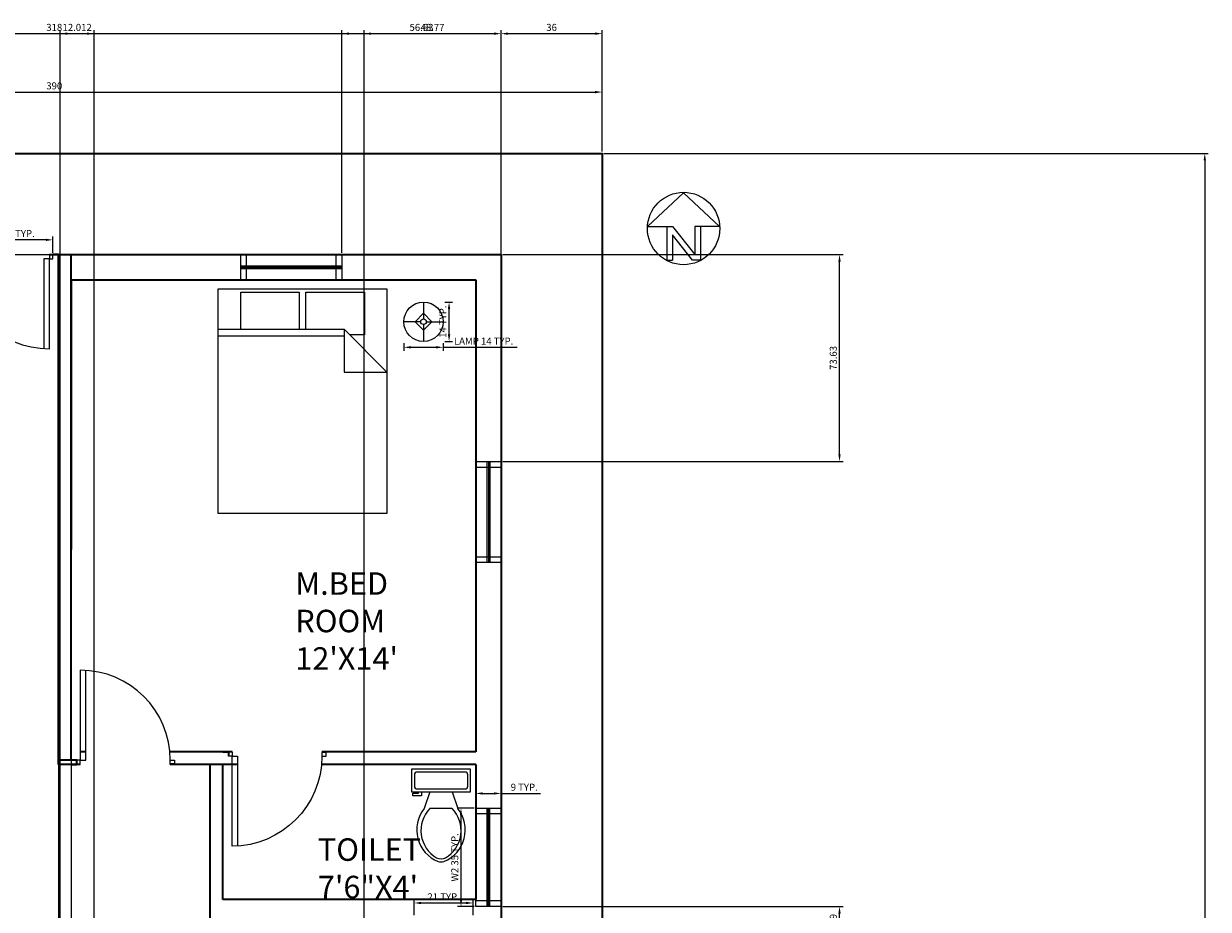
# Model space of a CAD drawing. Units: inches. Extents: x 204 to 942, y 1794 to 2670.
# Tile 6 of 6: x 521 to 942, y 2355 to 2670. Entities that reach past the tile are written whole.
import ezdxf

# ---------------------------------------------------------------- set-up
doc = ezdxf.new("R2010")
doc.units = ezdxf.units.IN
for name, color, linetype, lineweight in [('A-ANNO-DIMS', 2, 'Continuous', 18), ('A-ANNO-SYMB', 7, 'Continuous', 25), ('A-AREA-IDEN', 7, 'Continuous', 18), ('A-DOOR', 3, 'Continuous', 18), ('A-FLOR-FIXT', 9, 'Continuous', 18), ('A-FLOR-OTLN', 7, 'Continuous', 25), ('A-FURN', 8, 'Continuous', 18), ('A-GLAZ', 4, 'Continuous', 18), ('A-WALL', 7, 'Continuous', 35), ('C-PROP', 7, 'Continuous', 35)]:
    doc.layers.add(name, color=color, linetype=linetype, lineweight=lineweight)
doc.styles.get("Standard").update_dxf_attribs({"font": 'arial.ttf'})
doc.dimstyles.new('ISO-25', dxfattribs={"dimtxt": 2.5, "dimasz": 2.5, "dimexe": 1.25, "dimexo": 0.625, "dimtad": 1, "dimtxsty": 'Standard', "dimcen": 2.5, "dimadec": 0, "dimazin": 0, "dimtfac": 1, "dimtmove": 0, "dimatfit": 3, "dimfxl": 1, "dimarcsym": 0})

# ---------------------------------------------------------------- blocks, each defined once
blk = doc.blocks.new('Bed - Queen')
for p, q in [((0, -80.00003), (0, 0)), ((0, 0), (59.99999, 0)), ((59.99999, 0), (59.99999, -80.00003)), ((7.99999, -1.2), (28.79998, -1.2)), ((7.99999, -14.4), (7.99999, -1.2)), ((28.79998, -1.2), (28.79998, -14.4)), ((31.19999, -1.2), (51.99999, -1.2)), ((31.19999, -14.4), (31.19999, -1.2)), ((51.99999, -1.2), (51.99999, -16.4)), ((0, -14.4), (44.8, -14.4)), ((44.8, -16.8), (0, -16.8)), ((59.99999, -29.6), (44.8, -14.4)), ((44.8, -14.4), (44.8, -29.6)), ((51.99999, -16.4), (46.79936, -16.4)), ((44.8, -29.6), (59.99999, -29.6)), ((59.99999, -80.00003), (0, -80.00003))]:
    blk.add_line(p, q)
blk = doc.blocks.new('Lamp - Table')
for p, q in [((0, 7), (0, 1)), ((-1, 0), (-7, 0)), ((0, 3), (-3, 0)), ((-3, 0), (0, -3)), ((3, 0), (0, 3)), ((0, -3), (3, 0)), ((1, 0), (7, 0)), ((0, -1), (0, -7))]:
    blk.add_line(p, q)
for radius in [7, 1]:
    blk.add_circle((0, 0), radius)
blk = doc.blocks.new('Toilet - top')
for p, q in [((9.5, -6), (9.5, -2)), ((-8, -8.5), (-8, -8)), ((-7, -8), (-7, -9.5)), ((-4, -8), (-6, -14)), ((4, -8), (6, -14)), ((-10, -8.5), (-8, -8.5)), ((-10, -9.5), (-10, -8.5)), ((-7, -9.5), (-10, -9.5)), ((4, -14), (-4, -14))]:
    blk.add_line(p, q)
blk.add_lwpolyline([(10.5, -8), (10.5, 0), (-10.5, 0), (-10.5, -8)], close=True)
for points in [[(-9.5, -2), (-9.5, -6)], [(8.5, -1), (-8.5, -1)], [(-8.5, -7), (8.5, -7)]]:
    blk.add_lwpolyline(points)
for centre, radius, start, end in [((-8.62, -1.88), 0.884, 81.8699, 188.1301), ((8.62, -1.88), 0.884, 351.8699, 98.1301), ((-8.62, -6.12), 0.884, 171.8699, 278.1301), ((8.62, -6.12), 0.884, 261.8699, 8.1301), ((3.52, -21.58), 12.17, 141.4691, 247.9714), ((4.2, -21.82), 11.33, 136.3677, 238.9468), ((-3.52, -21.58), 12.17, 292.0284, 38.5307), ((-4.2, -21.82), 11.33, 301.053, 43.6321), ((0, -27.88), 4, 245.7318, 294.2682), ((0, -29), 4, 254.8605, 285.1395)]:
    blk.add_arc(centre, radius, start, end)
blk = doc.blocks.new('North Arrow')
for p, q in [((0, 0), (-12.86, -11.999)), ((0, 0), (12.782, -11.999)), ((-12.86, -11.999), (-6, -11.999)), ((-6, -11.999), (-6, -23.999)), ((-6, -11.999), (-4, -11.999)), ((-4, -11.999), (4, -21.999)), ((4, -11.999), (4, -21.999)), ((6, -11.999), (4, -11.999)), ((12.782, -11.999), (6, -11.999)), ((6, -11.999), (6, -23.999)), ((3.195, -23.996), (-4, -15.002)), ((-4, -15.002), (-4, -23.999)), ((-6, -23.999), (-4, -23.999)), ((6, -23.999), (3.195, -23.999))]:
    blk.add_line(p, q)
blk.add_circle((-0.013, -12.745), 12.885)
blk = doc.blocks.new('*D10')
at = {"layer": 'A-ANNO-DIMS', "color": 0, "lineweight": -2, "transparency": 16777216}
for p, q in [((336.74, 2624.88), (336.74, 2647.31)), ((339.24, 2646.06), (724.24, 2646.06)), ((726.74, 2624.88), (726.74, 2647.31))]:
    blk.add_line(p, q, dxfattribs=at)
at = {"layer": 'A-ANNO-DIMS', "color": 0, "transparency": 16777216}
for points in [[(339.24, 2646.47), (339.24, 2645.64), (336.74, 2646.06)], [(724.24, 2646.47), (724.24, 2645.64), (726.74, 2646.06)]]:
    blk.add_solid(points, dxfattribs=at)
at = {"layer": 'Defpoints', "color": 0, "transparency": 16777216}
for p in [(726.74, 2646.06), (336.74, 2624.26), (726.74, 2624.26)]:
    blk.add_point(p, dxfattribs=at)
at = {"layer": 'A-ANNO-DIMS', "color": 0, "transparency": 16777216, "insert": (531.74, 2647.96), "char_height": 2.5, "attachment_point": 5}
blk.add_mtext('390', dxfattribs=at)
blk = doc.blocks.new('*D12')
at = {"layer": 'A-ANNO-DIMS', "color": 0, "lineweight": -2, "transparency": 16777216}
for p, q in [((727.37, 2624.26), (942.46, 2624.26)), ((941.21, 2621.76), (941.21, 1840.76)), ((727.37, 1838.26), (942.46, 1838.26))]:
    blk.add_line(p, q, dxfattribs=at)
at = {"layer": 'A-ANNO-DIMS', "color": 0, "transparency": 16777216}
for points in [[(940.79, 2621.76), (941.63, 2621.76), (941.21, 2624.26)], [(940.79, 1840.76), (941.63, 1840.76), (941.21, 1838.26)]]:
    blk.add_solid(points, dxfattribs=at)
at = {"layer": 'Defpoints', "color": 0, "transparency": 16777216}
for p in [(726.74, 2624.26), (726.74, 1838.26), (941.21, 1838.26)]:
    blk.add_point(p, dxfattribs=at)
at = {"layer": 'A-ANNO-DIMS', "color": 0, "transparency": 16777216, "insert": (939.31, 2231.26), "char_height": 2.5, "attachment_point": 5, "rotation": 90}
blk.add_mtext('786', dxfattribs=at)
blk = doc.blocks.new('WIN-36IN')
for p, q in [((0, 9), (36, 9)), ((0, 0), (0, 9)), ((2, 0), (2, 9)), ((34, 0), (34, 9)), ((36, 9), (36, 0)), ((0, 5), (36, 5)), ((0, 4.5), (36, 4.5)), ((0, 4), (36, 4)), ((36, 0), (0, 0)), ((0, 0), (2, 0)), ((36, 0), (34, 0))]:
    blk.add_line(p, q)
blk = doc.blocks.new('WIN-35IN')
for p, q in [((0, 0), (0, 35)), ((0, 35), (9, 35)), ((4, 0), (4, 35)), ((4.5, 0), (4.5, 35)), ((5, 0), (5, 35)), ((9, 35), (9, 0)), ((9, 35), (9, 33)), ((9, 33), (0, 33)), ((9, 2), (0, 2)), ((9, 0), (0, 0)), ((9, 0), (9, 2))]:
    blk.add_line(p, q)
blk = doc.blocks.new('DOOR-SWING-32IN')
for p, q in [((3.26, 1.55), (3.26, 33.49)), ((1.26, 1.55), (3.26, 1.55))]:
    blk.add_line(p, q)
blk.add_lwpolyline([(1.26, 33.55), (1.26, 1.55), (3.26, 1.55)])
for points in [[(1.26, 1.55), (0, 1.55), (0, 0), (1.26, 0)], [(33.26, 1.55), (34.79, 1.55), (34.79, 0.26), (33.26, 0.26)]]:
    blk.add_lwpolyline(points, close=True)
blk.add_arc((1.26, 1.55), 32, 0, 90)
blk = doc.blocks.new('*D16')
at = {"layer": 'A-ANNO-DIMS', "color": 0, "lineweight": -2, "transparency": 16777216}
for p, q in [((496.46, 2588.88), (496.46, 2594.73)), ((528.74, 2593.48), (498.96, 2593.48)), ((531.24, 2588.88), (531.24, 2594.73))]:
    blk.add_line(p, q, dxfattribs=at)
at = {"layer": 'A-ANNO-DIMS', "color": 0, "transparency": 16777216}
for points in [[(498.96, 2593.89), (498.96, 2593.06), (496.46, 2593.48)], [(528.74, 2593.89), (528.74, 2593.06), (531.24, 2593.48)]]:
    blk.add_solid(points, dxfattribs=at)
at = {"layer": 'Defpoints', "color": 0, "transparency": 16777216}
for p in [(496.46, 2593.48), (496.46, 2588.26), (531.24, 2588.26)]:
    blk.add_point(p, dxfattribs=at)
at = {"layer": 'A-ANNO-DIMS', "color": 0, "transparency": 16777216, "insert": (513.85, 2595.4), "char_height": 2.5, "attachment_point": 5}
blk.add_mtext('DOOR 35 TYP.', dxfattribs=at)
blk = doc.blocks.new('*D20')
at = {"layer": 'A-ANNO-DIMS', "color": 0, "lineweight": -2, "transparency": 16777216}
for p, q in [((681.13, 2391.22), (675.26, 2391.22)), ((676.51, 2358.72), (676.51, 2388.72)), ((681.13, 2356.22), (675.26, 2356.22))]:
    blk.add_line(p, q, dxfattribs=at)
at = {"layer": 'A-ANNO-DIMS', "color": 0, "transparency": 16777216}
for points in [[(676.09, 2388.72), (676.92, 2388.72), (676.51, 2391.22)], [(676.09, 2358.72), (676.92, 2358.72), (676.51, 2356.22)]]:
    blk.add_solid(points, dxfattribs=at)
at = {"layer": 'Defpoints', "color": 0, "transparency": 16777216}
for p in [(676.51, 2391.22), (681.76, 2391.22), (681.76, 2356.22)]:
    blk.add_point(p, dxfattribs=at)
at = {"layer": 'A-ANNO-DIMS', "color": 0, "transparency": 16777216, "insert": (674.6, 2373.72), "char_height": 2.5, "attachment_point": 5, "rotation": 90}
blk.add_mtext('W2 35 TYP.', dxfattribs=at)
blk = doc.blocks.new('*D21')
at = {"layer": 'A-ANNO-DIMS', "color": 0, "lineweight": -2, "transparency": 16777216}
for p, q in [((681.76, 2391.85), (681.76, 2397.72)), ((684.26, 2396.47), (688.26, 2396.47)), ((690.76, 2391.85), (690.76, 2397.72)), ((690.76, 2396.47), (704.73, 2396.47))]:
    blk.add_line(p, q, dxfattribs=at)
at = {"layer": 'A-ANNO-DIMS', "color": 0, "transparency": 16777216}
for points in [[(684.26, 2396.89), (684.26, 2396.05), (681.76, 2396.47)], [(688.26, 2396.89), (688.26, 2396.05), (690.76, 2396.47)]]:
    blk.add_solid(points, dxfattribs=at)
at = {"layer": 'Defpoints', "color": 0, "transparency": 16777216}
for p in [(690.76, 2396.47), (681.76, 2391.22), (690.76, 2391.22)]:
    blk.add_point(p, dxfattribs=at)
at = {"layer": 'A-ANNO-DIMS', "color": 0, "transparency": 16777216, "insert": (698.99, 2398.37), "char_height": 2.5, "attachment_point": 5}
blk.add_mtext('9 TYP.', dxfattribs=at)
blk = doc.blocks.new('*D24')
at = {"layer": 'A-ANNO-DIMS', "color": 0, "lineweight": -2, "transparency": 16777216}
for p, q in [((656.15, 2556.71), (656.15, 2553.99)), ((658.65, 2555.24), (667.65, 2555.24)), ((670.15, 2556.71), (670.15, 2553.99)), ((670.15, 2555.24), (696.44, 2555.24))]:
    blk.add_line(p, q, dxfattribs=at)
at = {"layer": 'A-ANNO-DIMS', "color": 0, "transparency": 16777216}
for points in [[(658.65, 2555.65), (658.65, 2554.82), (656.15, 2555.24)], [(667.65, 2555.65), (667.65, 2554.82), (670.15, 2555.24)]]:
    blk.add_solid(points, dxfattribs=at)
at = {"layer": 'Defpoints', "color": 0, "transparency": 16777216}
for p in [(656.15, 2557.34), (670.15, 2557.34), (670.15, 2555.24)]:
    blk.add_point(p, dxfattribs=at)
at = {"layer": 'A-ANNO-DIMS', "color": 0, "transparency": 16777216, "insert": (684.54, 2557.12), "char_height": 2.5, "attachment_point": 5}
blk.add_mtext('LAMP 14 TYP.', dxfattribs=at)
blk = doc.blocks.new('*D25')
at = {"layer": 'A-ANNO-DIMS', "color": 0, "lineweight": -2, "transparency": 16777216}
for p, q in [((670.77, 2571.34), (673.5, 2571.34)), ((672.25, 2559.84), (672.25, 2568.84)), ((670.77, 2557.34), (673.5, 2557.34))]:
    blk.add_line(p, q, dxfattribs=at)
at = {"layer": 'A-ANNO-DIMS', "color": 0, "transparency": 16777216}
for points in [[(671.83, 2568.84), (672.67, 2568.84), (672.25, 2571.34)], [(671.83, 2559.84), (672.67, 2559.84), (672.25, 2557.34)]]:
    blk.add_solid(points, dxfattribs=at)
at = {"layer": 'Defpoints', "color": 0, "transparency": 16777216}
for p in [(670.15, 2571.34), (672.25, 2571.34), (670.15, 2557.34)]:
    blk.add_point(p, dxfattribs=at)
at = {"layer": 'A-ANNO-DIMS', "color": 0, "transparency": 16777216, "insert": (670.37, 2564.34), "char_height": 2.5, "attachment_point": 5, "rotation": 90}
blk.add_mtext('14 TYP.', dxfattribs=at)
blk = doc.blocks.new('*D27')
at = {"layer": 'A-ANNO-DIMS', "color": 0, "lineweight": -2, "transparency": 16777216}
for p, q in [((659.8, 2353.16), (659.8, 2358.74)), ((662.3, 2357.49), (678.3, 2357.49)), ((680.8, 2353.16), (680.8, 2358.74))]:
    blk.add_line(p, q, dxfattribs=at)
at = {"layer": 'A-ANNO-DIMS', "color": 0, "transparency": 16777216}
for points in [[(662.3, 2357.91), (662.3, 2357.07), (659.8, 2357.49)], [(678.3, 2357.91), (678.3, 2357.07), (680.8, 2357.49)]]:
    blk.add_solid(points, dxfattribs=at)
at = {"layer": 'Defpoints', "color": 0, "transparency": 16777216}
for p in [(680.8, 2357.49), (659.8, 2352.53), (680.8, 2352.53)]:
    blk.add_point(p, dxfattribs=at)
at = {"layer": 'A-ANNO-DIMS', "color": 0, "transparency": 16777216, "insert": (670.3, 2359.37), "char_height": 2.5, "attachment_point": 5}
blk.add_mtext('21 TYP.', dxfattribs=at)
blk = doc.blocks.new('*D38')
at = {"layer": 'A-ANNO-DIMS', "color": 0, "lineweight": -2, "transparency": 16777216}
for p, q in [((372.74, 2624.88), (372.74, 2668.11)), ((375.24, 2666.86), (688.24, 2666.86)), ((690.74, 2624.88), (690.74, 2668.11))]:
    blk.add_line(p, q, dxfattribs=at)
at = {"layer": 'A-ANNO-DIMS', "color": 0, "transparency": 16777216}
for points in [[(375.24, 2667.28), (375.24, 2666.44), (372.74, 2666.86)], [(688.24, 2667.28), (688.24, 2666.44), (690.74, 2666.86)]]:
    blk.add_solid(points, dxfattribs=at)
at = {"layer": 'Defpoints', "color": 0, "transparency": 16777216}
for p in [(690.74, 2666.86), (372.74, 2624.26), (690.74, 2624.26)]:
    blk.add_point(p, dxfattribs=at)
at = {"layer": 'A-ANNO-DIMS', "color": 0, "transparency": 16777216, "insert": (531.74, 2668.76), "char_height": 2.5, "attachment_point": 5}
blk.add_mtext('318', dxfattribs=at)
blk = doc.blocks.new('*D41')
at = {"layer": 'A-ANNO-DIMS', "color": 0, "lineweight": -2, "transparency": 16777216}
for p, q in [((690.74, 2588.88), (690.74, 2668.11)), ((693.24, 2666.86), (724.24, 2666.86)), ((726.74, 2624.88), (726.74, 2668.11))]:
    blk.add_line(p, q, dxfattribs=at)
at = {"layer": 'A-ANNO-DIMS', "color": 0, "transparency": 16777216}
for points in [[(693.24, 2667.28), (693.24, 2666.44), (690.74, 2666.86)], [(724.24, 2667.28), (724.24, 2666.44), (726.74, 2666.86)]]:
    blk.add_solid(points, dxfattribs=at)
at = {"layer": 'Defpoints', "color": 0, "transparency": 16777216}
for p in [(726.74, 2666.86), (726.74, 2624.26), (690.74, 2588.26)]:
    blk.add_point(p, dxfattribs=at)
at = {"layer": 'A-ANNO-DIMS', "color": 0, "transparency": 16777216, "insert": (708.74, 2668.76), "char_height": 2.5, "attachment_point": 5}
blk.add_mtext('36', dxfattribs=at)
blk = doc.blocks.new('*D47')
at = {"layer": 'A-ANNO-DIMS', "color": 0, "lineweight": -2, "transparency": 16777216}
for p, q in [((533.86, 2137.88), (533.86, 2668.11)), ((536.36, 2666.86), (543.38, 2666.86)), ((545.88, 2137.88), (545.88, 2668.11))]:
    blk.add_line(p, q, dxfattribs=at)
at = {"layer": 'A-ANNO-DIMS', "color": 0, "transparency": 16777216}
for points in [[(536.36, 2667.28), (536.36, 2666.44), (533.86, 2666.86)], [(543.38, 2667.28), (543.38, 2666.44), (545.88, 2666.86)]]:
    blk.add_solid(points, dxfattribs=at)
at = {"layer": 'Defpoints', "color": 0, "transparency": 16777216}
for p in [(545.88, 2666.86), (533.86, 2137.26), (545.88, 2137.26)]:
    blk.add_point(p, dxfattribs=at)
at = {"layer": 'A-ANNO-DIMS', "color": 0, "transparency": 16777216, "insert": (539.87, 2668.76), "char_height": 2.5, "attachment_point": 5}
blk.add_mtext('12.012', dxfattribs=at)
blk = doc.blocks.new('*D48')
at = {"layer": 'A-ANNO-DIMS', "color": 0, "lineweight": -2, "transparency": 16777216}
for p, q in [((641.98, 2014.8), (641.98, 2668.11)), ((644.48, 2666.86), (688.24, 2666.86)), ((690.74, 2014.8), (690.74, 2668.11))]:
    blk.add_line(p, q, dxfattribs=at)
at = {"layer": 'A-ANNO-DIMS', "color": 0, "transparency": 16777216}
for points in [[(644.48, 2667.28), (644.48, 2666.44), (641.98, 2666.86)], [(688.24, 2667.28), (688.24, 2666.44), (690.74, 2666.86)]]:
    blk.add_solid(points, dxfattribs=at)
at = {"layer": 'Defpoints', "color": 0, "transparency": 16777216}
for p in [(690.74, 2666.86), (641.98, 2014.18), (690.74, 2014.18)]:
    blk.add_point(p, dxfattribs=at)
at = {"layer": 'A-ANNO-DIMS', "color": 0, "transparency": 16777216, "insert": (666.36, 2668.76), "char_height": 2.5, "attachment_point": 5}
blk.add_mtext('48.77', dxfattribs=at)
blk = doc.blocks.new('*D50')
at = {"layer": 'A-ANNO-DIMS', "color": 0, "lineweight": -2, "transparency": 16777216}
for p, q in [((533.24, 2587.63), (533.24, 1794.41)), ((537.74, 2578.63), (537.74, 1794.41)), ((530.74, 1795.66), (528.24, 1795.66)), ((533.24, 1795.66), (537.74, 1795.66)), ((540.24, 1795.66), (548.67, 1795.66))]:
    blk.add_line(p, q, dxfattribs=at)
at = {"layer": 'A-ANNO-DIMS', "color": 0, "transparency": 16777216}
for points in [[(530.74, 1796.08), (530.74, 1795.24), (533.24, 1795.66)], [(540.24, 1796.08), (540.24, 1795.24), (537.74, 1795.66)]]:
    blk.add_solid(points, dxfattribs=at)
at = {"layer": 'Defpoints', "color": 0, "transparency": 16777216}
for p in [(533.24, 2588.26), (537.74, 2579.26), (537.74, 1795.66)]:
    blk.add_point(p, dxfattribs=at)
at = {"layer": 'A-ANNO-DIMS', "color": 0, "transparency": 16777216, "insert": (545.7, 1797.56), "char_height": 2.5, "attachment_point": 5}
blk.add_mtext('4.5', dxfattribs=at)
blk = doc.blocks.new('*D53')
at = {"layer": 'A-ANNO-DIMS', "color": 0, "lineweight": -2, "transparency": 16777216}
for p, q in [((634.11, 2588.9), (634.11, 2668.11)), ((636.61, 2666.86), (688.24, 2666.86)), ((690.74, 2588.88), (690.74, 2668.11))]:
    blk.add_line(p, q, dxfattribs=at)
at = {"layer": 'A-ANNO-DIMS', "color": 0, "transparency": 16777216}
for points in [[(636.61, 2667.28), (636.61, 2666.44), (634.11, 2666.86)], [(688.24, 2667.28), (688.24, 2666.44), (690.74, 2666.86)]]:
    blk.add_solid(points, dxfattribs=at)
at = {"layer": 'Defpoints', "color": 0, "transparency": 16777216}
for p in [(690.74, 2666.86), (634.11, 2588.28), (690.74, 2588.26)]:
    blk.add_point(p, dxfattribs=at)
at = {"layer": 'A-ANNO-DIMS', "color": 0, "transparency": 16777216, "insert": (662.43, 2668.76), "char_height": 2.5, "attachment_point": 5}
blk.add_mtext('56.63', dxfattribs=at)
blk = doc.blocks.new('*D59')
at = {"layer": 'A-ANNO-DIMS', "color": 0, "lineweight": -2, "transparency": 16777216}
for p, q in [((691.37, 2588.26), (812.46, 2588.26)), ((811.21, 2517.13), (811.21, 2585.76)), ((691.35, 2514.63), (812.46, 2514.63))]:
    blk.add_line(p, q, dxfattribs=at)
at = {"layer": 'A-ANNO-DIMS', "color": 0, "transparency": 16777216}
for points in [[(810.79, 2585.76), (811.62, 2585.76), (811.21, 2588.26)], [(810.79, 2517.13), (811.62, 2517.13), (811.21, 2514.63)]]:
    blk.add_solid(points, dxfattribs=at)
at = {"layer": 'Defpoints', "color": 0, "transparency": 16777216}
for p in [(690.74, 2588.26), (811.21, 2588.26), (690.72, 2514.63)]:
    blk.add_point(p, dxfattribs=at)
at = {"layer": 'A-ANNO-DIMS', "color": 0, "transparency": 16777216, "insert": (809.31, 2551.45), "char_height": 2.5, "attachment_point": 5, "rotation": 90}
blk.add_mtext('73.63', dxfattribs=at)
blk = doc.blocks.new('*D61')
at = {"layer": 'A-ANNO-DIMS', "color": 0, "lineweight": -2, "transparency": 16777216}
for p, q in [((691.38, 2356.22), (812.46, 2356.22)), ((811.21, 2344.93), (811.21, 2353.72)), ((691.38, 2342.43), (812.46, 2342.43))]:
    blk.add_line(p, q, dxfattribs=at)
at = {"layer": 'A-ANNO-DIMS', "color": 0, "transparency": 16777216}
for points in [[(810.79, 2353.72), (811.62, 2353.72), (811.21, 2356.22)], [(810.79, 2344.93), (811.62, 2344.93), (811.21, 2342.43)]]:
    blk.add_solid(points, dxfattribs=at)
at = {"layer": 'Defpoints', "color": 0, "transparency": 16777216}
for p in [(690.76, 2356.22), (811.21, 2356.22), (690.75, 2342.43)]:
    blk.add_point(p, dxfattribs=at)
at = {"layer": 'A-ANNO-DIMS', "color": 0, "transparency": 16777216, "insert": (809.31, 2349.33), "char_height": 2.5, "attachment_point": 5, "rotation": 90}
blk.add_mtext('13.79', dxfattribs=at)

msp = doc.modelspace()

# ---------------------------------------------------------------- linework, layer by layer
at = {"layer": 'A-FLOR-OTLN'}
msp.add_lwpolyline([(372.7443, 2588.2597), (690.7443, 2588.2597), (690.7443, 2138.2597), (372.7443, 2138.2597)], close=True, dxfattribs=at)
at = {"layer": 'A-WALL'}
for p, q in [((529.9822, 2588.2597), (537.7443, 2588.2597)), ((533.2443, 2588.2597), (531.2443, 2588.2597)), ((533.2443, 2588.2597), (690.7443, 2588.2597)), ((533.2443, 2579.2597), (533.2443, 2588.2597)), ((537.7443, 2579.2597), (537.7443, 2588.2597)), ((537.7443, 2588.2597), (539.7443, 2588.2597)), ((539.7443, 2588.2597), (548.9949, 2588.2597)), ((690.7443, 2588.2597), (690.7443, 2411.2597)), ((533.2443, 2579.2597), (533.2443, 2483.2597)), ((533.2443, 2411.2597), (533.2443, 2579.2597)), ((537.7443, 2579.2597), (537.7443, 2483.2597)), ((537.7443, 2579.2597), (681.7443, 2579.2597)), ((537.7443, 2411.2597), (537.7443, 2579.2597)), ((681.7443, 2579.2597), (681.7443, 2411.2597)), ((533.2443, 2406.7597), (533.2443, 2478.7597)), ((533.2443, 2406.7597), (533.2443, 2478.7597)), ((537.7443, 2408.3112), (537.7443, 2478.7597)), ((537.7443, 2408.3112), (537.7443, 2478.7597)), ((539.7443, 2408.3112), (533.2443, 2408.3112)), ((539.7443, 2406.7597), (539.7443, 2408.3112)), ((543.0064, 2411.2597), (541.0064, 2411.2597)), ((595.0064, 2411.2597), (572.8703, 2411.2597)), ((591.7443, 2411.2597), (593.7443, 2411.2597)), ((593.7443, 2411.2597), (593.7443, 2409.7082)), ((681.7443, 2411.2597), (626.9688, 2411.2597)), ((690.7443, 2411.2597), (690.7443, 2330.2597)), ((537.7443, 2406.7597), (533.2443, 2406.7597)), ((537.7443, 2406.7597), (539.7443, 2406.7597)), ((541.0064, 2406.7597), (537.7443, 2406.7597)), ((573.0064, 2407.0155), (573.0064, 2406.7597)), ((597.0064, 2406.7597), (573.0064, 2406.7597)), ((587.2443, 2358.7597), (587.2443, 2406.7597)), ((591.7443, 2358.7597), (591.7443, 2406.7597)), ((681.7443, 2406.7597), (626.8703, 2406.7597)), ((681.7443, 2406.7597), (681.7443, 2358.7597)), ((587.2443, 2341.4841), (587.2443, 2358.7597)), ((681.7443, 2358.7597), (591.7443, 2358.7597)), ((681.7443, 2358.7597), (591.7443, 2358.7597))]:
    msp.add_line(p, q, dxfattribs=at)
at = {"layer": 'C-PROP'}
for p, q in [((533.2443, 2624.2597), (690.7443, 2624.2597)), ((726.7443, 2588.2597), (726.7443, 2411.2597))]:
    msp.add_line(p, q, dxfattribs=at)
msp.add_lwpolyline([(336.7443, 2102.2597), (336.7443, 2624.2597), (726.7443, 2624.2597), (726.7443, 2102.2597)], dxfattribs=at)

# ---------------------------------------------------------------- block references
at = {"layer": 'A-ANNO-SYMB'}
msp.add_blockref('North Arrow', (755.7363, 2610.2578), dxfattribs=at)
at = {"layer": 'A-DOOR', "rotation": 180}
msp.add_blockref('DOOR-SWING-32IN', (531.2446, 2588.2593), dxfattribs=at)
at = {"layer": 'A-DOOR'}
msp.add_blockref('DOOR-SWING-32IN', (539.744, 2406.76), dxfattribs=at)
at = {"layer": 'A-DOOR', "extrusion": (0, 0, -1), "zscale": -1, "rotation": 180}
msp.add_blockref('DOOR-SWING-32IN', (-593.744, 2411.2593), dxfattribs=at)
at = {"layer": 'A-FLOR-FIXT'}
msp.add_blockref('Toilet - top', (669.3848, 2405.0832), dxfattribs=at)
at = {"layer": 'A-FURN'}
for name, p in [('Bed - Queen', (590.1138, 2576.0464)), ('Lamp - Table', (663.1483, 2564.3369))]:
    msp.add_blockref(name, p, dxfattribs=at)
at = {"layer": 'A-GLAZ'}
for name, p in [('WIN-36IN', (598.1145, 2579.2787)), ('WIN-35IN', (681.756, 2356.22))]:
    msp.add_blockref(name, p, dxfattribs=at)
at = {"layer": 'A-GLAZ', "rotation": 269.9999999999968}
msp.add_blockref('WIN-36IN', (681.7224, 2514.6308), dxfattribs=at)

# ---------------------------------------------------------------- texts
at = {"layer": 'A-AREA-IDEN', "char_height": 2.5, "attachment_point": 1}
for s, insert in [("{\\H3.2x;M.BED ROOM\\P12'X14'   }", (617.5185, 2475.1677)), ('{\\H3.2x;TOILET\\P7\'6"X4\' }', (625.5563, 2380.4915))]:
    msp.add_mtext_dynamic_manual_height_columns(s, width=46.676204, gutter_width=12.5, heights=[0], dxfattribs=dict(at, insert=insert))

# ---------------------------------------------------------------- dimensions: what is measured, and where the dimension line sits
at = {"layer": 'A-ANNO-DIMS'}
for base, p1, p2, override, picture, middle in [((690.7443, 2666.8597), (372.7443, 2624.2597), (690.7443, 2624.2597), {"dimdec": 0, "dimlfac": 1, "dimrnd": 0, "dimzin": 0, "dimdsep": 46, "dimlunit": 2}, '*D38', (531.7443, 2668.7619)), ((545.8757, 2666.8597), (533.8633, 2137.2597), (545.8757, 2137.2597), {"dimdec": 3, "dimlfac": 1, "dimrnd": 0, "dimzin": 0, "dimdsep": 46, "dimlunit": 2}, '*D47', (539.8695, 2668.7611)), ((690.7443, 2666.8597), (634.114, 2588.2789), (690.7443, 2588.2597), {"dimdec": 2, "dimlfac": 1, "dimrnd": 0, "dimzin": 0, "dimdsep": 46, "dimlunit": 2}, '*D53', (662.4291, 2668.7619)), ((690.7443, 2666.8597), (641.9756, 2014.1774), (690.7443, 2014.1774), {"dimdec": 2, "dimlfac": 1, "dimrnd": 0, "dimzin": 0, "dimdsep": 46, "dimlunit": 2}, '*D48', (666.3599, 2668.7611)), ((726.7443, 2666.8597), (690.7443, 2588.2597), (726.7443, 2624.2597), {"dimdec": 0, "dimlfac": 1, "dimrnd": 0, "dimzin": 0, "dimdsep": 46, "dimlunit": 2}, '*D41', (708.7443, 2668.7619)), ((726.7443, 2646.0578), (336.7443, 2624.2597), (726.7443, 2624.2597), {"dimclrd": 0, "dimclre": 0, "dimclrt": 0}, '*D10', (531.7443, 2647.9601)), ((537.7443, 1795.6597), (533.2443, 2588.2597), (537.7443, 2579.2597), {"dimdec": 1, "dimlfac": 1, "dimrnd": 0, "dimzin": 0, "dimdsep": 46, "dimlunit": 2}, '*D50', (545.7047, 1797.556))]:
    dim = msp.add_linear_dim(base=base, p1=p1, p2=p2, dimstyle='ISO-25', override=override, dxfattribs=at)
    dim.commit()
    dim.dimension.update_dxf_attribs({"geometry": picture, "text_midpoint": middle})
for base, p1, p2, override, picture, middle in [((941.2084, 1838.2597), (726.7443, 2624.2597), (726.7443, 1838.2597), {"dimclrd": 0, "dimclre": 0, "dimclrt": 0}, '*D12', (939.307, 2231.2597)), ((811.2079, 2588.2597), (690.7226, 2514.6313), (690.7443, 2588.2597), {"dimdec": 2, "dimlfac": 1, "dimrnd": 0, "dimzin": 0, "dimdsep": 46, "dimlunit": 2}, '*D59', (809.3056, 2551.4455)), ((811.2079, 2356.22), (690.7515, 2342.4314), (690.756, 2356.22), {"dimdec": 2, "dimlfac": 1, "dimrnd": 0, "dimzin": 0, "dimdsep": 46, "dimlunit": 2}, '*D61', (809.3056, 2349.3257))]:
    dim = msp.add_linear_dim(base=base, p1=p1, p2=p2, angle=90, dimstyle='ISO-25', override=override, dxfattribs=at)
    dim.commit()
    dim.dimension.update_dxf_attribs({"geometry": picture, "text_midpoint": middle})
for base, p1, p2, angle, text, picture, middle in [((496.4586, 2593.4775), (531.2443, 2588.2597), (496.4586, 2588.2597), 180, 'DOOR <> TYP.', '*D16', (513.8515, 2595.3969)), ((672.2483, 2571.3369), (670.1483, 2557.3369), (670.1483, 2571.3369), 90, '<> TYP.', '*D25', (670.3674, 2564.3369)), ((676.506, 2391.22), (681.756, 2356.22), (681.756, 2391.22), 90, 'W2 <> TYP.', '*D20', (674.6037, 2373.72))]:
    dim = msp.add_linear_dim(base=base, p1=p1, p2=p2, angle=angle, text=text, dimstyle='ISO-25', override={"dimdec": 0, "dimlfac": 1, "dimrnd": 0, "dimzin": 0, "dimdsep": 46, "dimlunit": 2}, dxfattribs=at)
    dim.commit()
    dim.dimension.update_dxf_attribs({"geometry": picture, "text_midpoint": middle})
for base, p1, p2, text, picture, middle in [((670.1483, 2555.2369), (656.1483, 2557.3369), (670.1483, 2557.3369), 'LAMP <> TYP.', '*D24', (684.5429, 2557.1179)), ((690.756, 2396.47), (681.756, 2391.22), (690.756, 2391.22), '<> TYP.', '*D21', (698.9944, 2398.3715)), ((680.8042, 2357.4898), (659.8042, 2352.5328), (680.8042, 2352.5328), '<> TYP.', '*D27', (670.3042, 2359.3707))]:
    dim = msp.add_linear_dim(base=base, p1=p1, p2=p2, text=text, dimstyle='ISO-25', override={"dimdec": 0, "dimlfac": 1, "dimrnd": 0, "dimzin": 0, "dimdsep": 46, "dimlunit": 2}, dxfattribs=at)
    dim.commit()
    dim.dimension.update_dxf_attribs({"geometry": picture, "text_midpoint": middle})

doc.saveas('drawing.dxf')
